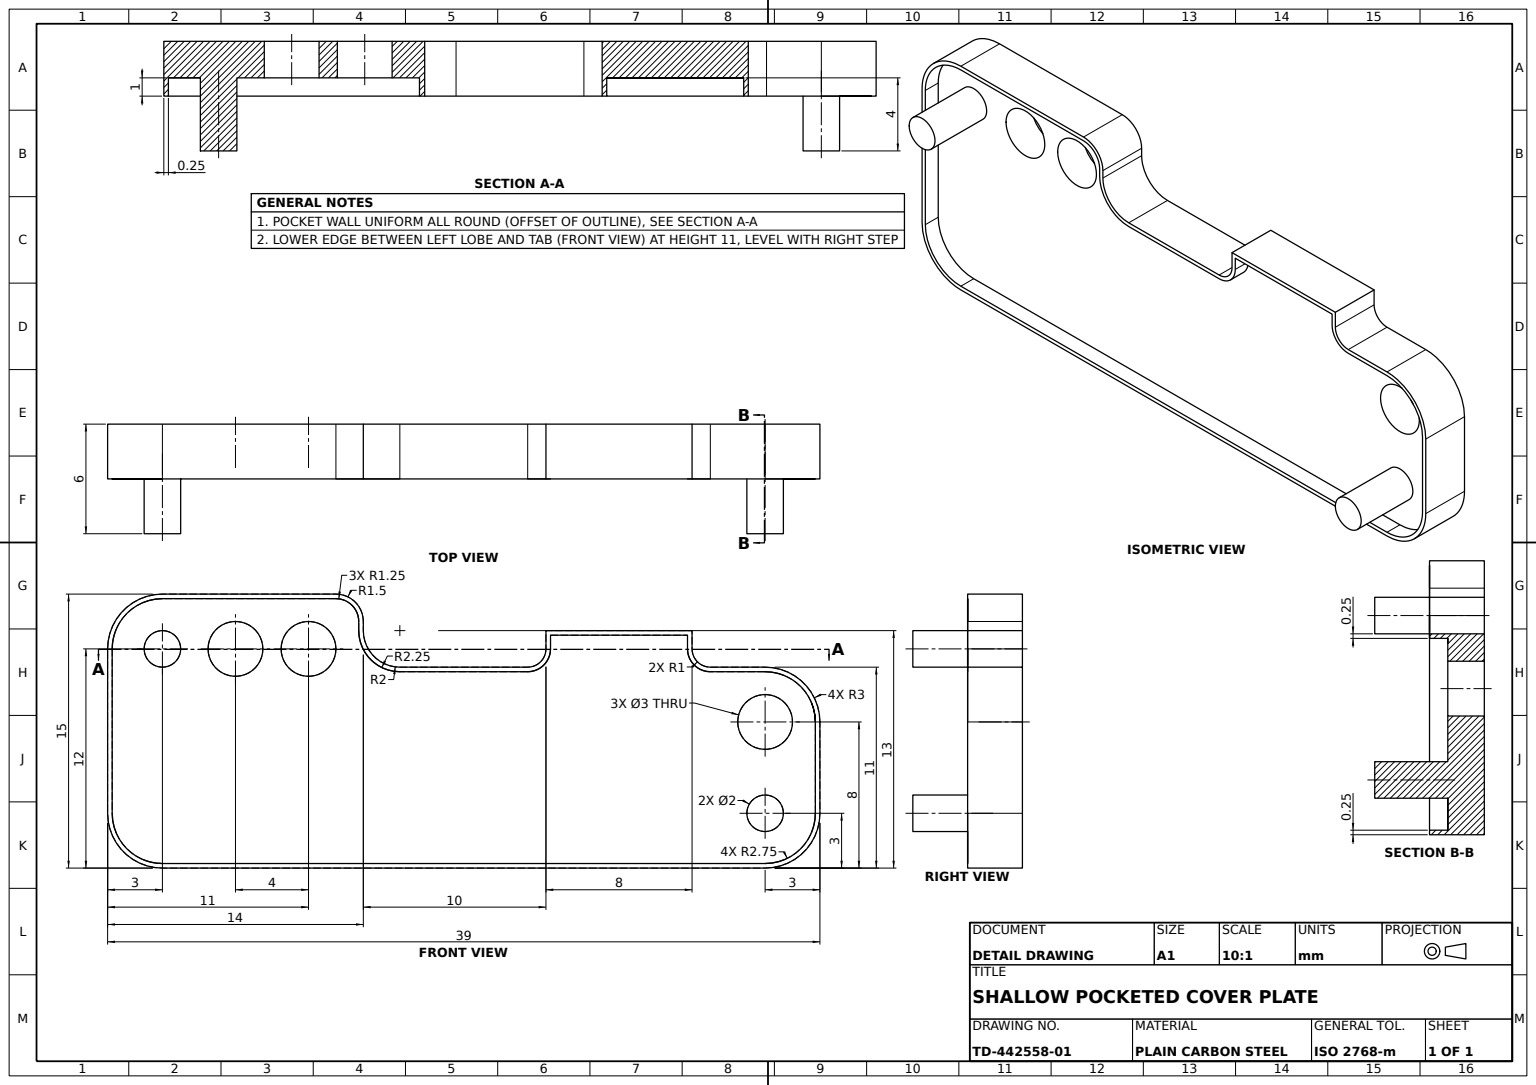
SolidWorks part; units mm, degrees
material "Plain Carbon Steel"
ref_plane "Front Plane" through (0, 0, 0) normal (0, 0, 1) x (1, 0, 0)
ref_plane "Top Plane" through (0, 0, 0) normal (0, 1, 0) x (1, 0, 0)
ref_plane "Right Plane" through (0, 0, 0) normal (1, 0, 0) x (0, 0, -1)
sketch "Plate Outline Sketch" plane through (0, 0, 0) normal (0, 0, 1) x (1, 0, 0)
  line L0 (4.5, 5.5) -> (12.5, 5.5)
  line L1 (-16.5, 7.5) -> (-7, 7.5)
  line L2 (-19.5, 4.5) -> (-19.5, -4.5)
  line L3 (-16.5, -7.5) -> (16.5, -7.5)
  line L4 (19.5, 0.5) -> (19.5, -4.5)
  line L7 (-3.5, 3.5) -> (3.5, 3.5)
  line L8 (-5.5, 5.5) -> (-5.5, 6)
  line L10 (4.5, 4.5) -> (4.5, 5.5)
  line L13 (13.5, 3.5) -> (16.5, 3.5)
  line L14 (12.5, 4.5) -> (12.5, 5.5)
  arc A0 (-3.5, 3.5) -> (-5.5, 5.5) centre (-3.5, 5.5) cw
  arc A1 (16.5, -7.5) -> (19.5, -4.5) centre (16.5, -4.5) ccw
  arc A2 (-19.5, -4.5) -> (-16.5, -7.5) centre (-16.5, -4.5) ccw
  arc A3 (-16.5, 7.5) -> (-19.5, 4.5) centre (-16.5, 4.5) ccw
  arc A4 (16.5, 3.5) -> (19.5, 0.5) centre (16.5, 0.5) cw
  arc A5 (3.5, 3.5) -> (4.5, 4.5) centre (3.5, 4.5) ccw
  arc A6 (12.5, 4.5) -> (13.5, 3.5) centre (13.5, 4.5) ccw
  arc A7 (-5.5, 6) -> (-7, 7.5) centre (-7, 6) ccw
  circle A8 centre (-16.5, 4.5) radius 1
  circle A9 centre (-12.5, 4.5) radius 1.5
  circle A10 centre (-8.5, 4.5) radius 1.5
  circle A11 centre (16.5, 0.5) radius 1.5
  circle A12 centre (16.5, -4.5) radius 1
  point P0 (0, 0)
  point P6 (-2.9165, 4.7583)
  point P23 (-19.5, -7.5)
  point P26 (-19.5, 7.5)
  dimension "D2" = 2
  dimension "D3" = 3
  dimension "D9" = 3
  dimension "D10" = 3
  dimension "D11" = 2
  dimension "D12" = 2
  dimension "D13" = 1
  dimension "D15" = 1.5
  dimension "D20" = 2
  dimension "D21" = 3
  dimension "D22" = 3
  dimension "D23" = 3
  dimension "D24" = 2
  dimension "D1" = 15
  dimension "D4" = 7
  dimension "D5" = 2
  dimension "D6" = 2
  dimension "D7" = 13
  dimension "D8" = 10
  dimension "D14" = 39
  dimension "D16" = 14
  dimension "D17" = 4
  dimension "D18" = 7
  dimension "D19" = 4
  dimension "D25" = 19.5
  dimension "D26" = 7.5
  dimension "D27" = 2.9165
  dimension "D28" = 4.7583
extrude "Base Plate 3mm" add sketch "Plate Outline Sketch" along normal blind 3
sketch "Pocket Outline Sketch" plane through (0, 0, 3) normal (0, 0, 1) x (1, 0, 0)
  line L20 (16.5, 3.25) -> (13.5, 3.25)
  line L21 (12.25, 4.5) -> (12.25, 5.25)
  line L22 (12.25, 5.25) -> (4.75, 5.25)
  line L23 (4.75, 5.25) -> (4.75, 4.5)
  line L24 (3.5, 3.25) -> (-3.5, 3.25)
  line L25 (-5.75, 5.5) -> (-5.75, 6)
  line L26 (-7, 7.25) -> (-16.5, 7.25)
  line L27 (-19.25, 4.5) -> (-19.25, -4.5)
  line L28 (-16.5, -7.25) -> (16.5, -7.25)
  line L29 (19.25, -4.5) -> (19.25, 0.5)
  line L30 (16.5, 3.25) -> (13.5, 3.25)
  line L31 (12.25, 4.5) -> (12.25, 5.25)
  line L32 (12.25, 5.25) -> (4.75, 5.25)
  line L33 (4.75, 5.25) -> (4.75, 4.5)
  line L34 (3.5, 3.25) -> (-3.5, 3.25)
  line L35 (-5.75, 5.5) -> (-5.75, 6)
  line L36 (-7, 7.25) -> (-16.5, 7.25)
  line L37 (-19.25, 4.5) -> (-19.25, -4.5)
  line L38 (-16.5, -7.25) -> (16.5, -7.25)
  line L39 (19.25, -4.5) -> (19.25, 0.5)
  arc A16 (19.25, 0.5) -> (16.5, 3.25) centre (16.5, 0.5) ccw
  arc A17 (12.25, 4.5) -> (13.5, 3.25) centre (13.5, 4.5) ccw
  arc A18 (3.5, 3.25) -> (4.75, 4.5) centre (3.5, 4.5) ccw
  arc A19 (-5.75, 5.5) -> (-3.5, 3.25) centre (-3.5, 5.5) ccw
  arc A20 (-5.75, 6) -> (-7, 7.25) centre (-7, 6) ccw
  arc A21 (-16.5, 7.25) -> (-19.25, 4.5) centre (-16.5, 4.5) ccw
  arc A22 (-19.25, -4.5) -> (-16.5, -7.25) centre (-16.5, -4.5) ccw
  arc A23 (16.5, -7.25) -> (19.25, -4.5) centre (16.5, -4.5) ccw
  arc A24 (19.25, 0.5) -> (16.5, 3.25) centre (16.5, 0.5) ccw
  arc A25 (12.25, 4.5) -> (13.5, 3.25) centre (13.5, 4.5) ccw
  arc A26 (3.5, 3.25) -> (4.75, 4.5) centre (3.5, 4.5) ccw
  arc A27 (-5.75, 5.5) -> (-3.5, 3.25) centre (-3.5, 5.5) ccw
  arc A28 (-5.75, 6) -> (-7, 7.25) centre (-7, 6) ccw
  arc A29 (-16.5, 7.25) -> (-19.25, 4.5) centre (-16.5, 4.5) ccw
  arc A30 (-19.25, -4.5) -> (-16.5, -7.25) centre (-16.5, -4.5) ccw
  arc A31 (16.5, -7.25) -> (19.25, -4.5) centre (16.5, -4.5) ccw
  dimension "D1" = 0.25
extrude "Recess Pocket 1mm" cut sketch "Pocket Outline Sketch" against normal blind 1 and the other way through all
sketch "Locating Pin Sketch" plane through (0, 0, 0) normal (0, 0, -1) x (-1, 0, 0)
  circle A0 centre (16.5, 4.5) radius 1 construction
  circle A1 centre (-16.5, -4.5) radius 1 construction
  circle A2 centre (16.5, 4.5) radius 1
  circle A3 centre (-16.5, -4.5) radius 1
extrude "Locating Pins 2x" add sketch "Locating Pin Sketch" against normal blind 6
